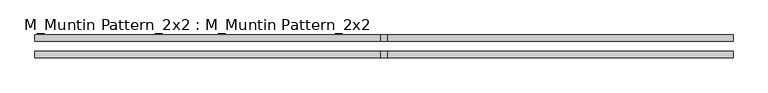
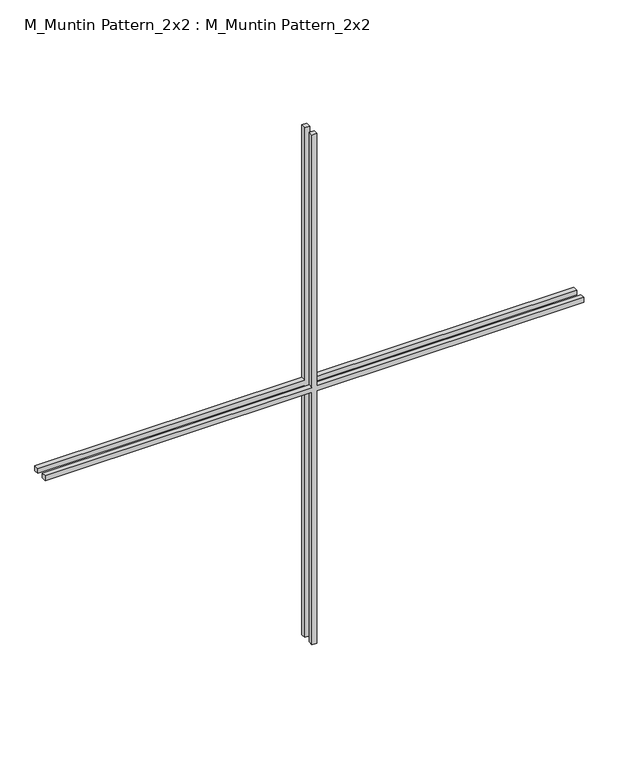
"""IFC4 building model written with IfcOpenShell, lengths in millimetres: proxy geometry, M_Muntin Pattern_2x2 : M_Muntin Pattern_2x2."""

from ifc_helpers import new_model, si_unit, frame, origin, place, context, project, spatial, polyline, outline, extrude, source, transform, mapped, element, save


def m_muntin_pattern_2x2_m_muntin_pattern_2x2_c1fd4460(model_context):
    return source(origin(), model_context, "Body", "SweptSolid", [
        extrude(outline(polyline([(686.5, -6.35), (686.5, -680.15), (673.8, -680.15), (673.8, -6.35), (0.0, -6.35), (0.0, 6.35), (673.8, 6.35), (673.8, 680.15), (686.5, 680.15), (686.5, 6.35), (1360.3, 6.35), (1360.3, -6.35), (686.5, -6.35)])), frame((0.0, 9.525, 0.0), z_axis=(0.0, 1.0, 0.0), x_axis=(0.0, 0.0, 1.0)), (0.0, 0.0, 1.0), 12.7),
        extrude(outline(polyline([(686.5, -6.35), (686.5, -680.15), (673.8, -680.15), (673.8, -6.35), (0.0, -6.35), (0.0, 6.35), (673.8, 6.35), (673.8, 680.15), (686.5, 680.15), (686.5, 6.35), (1360.3, 6.35), (1360.3, -6.35), (686.5, -6.35)])), frame((0.0, -22.225, 0.0), z_axis=(0.0, 1.0, 0.0), x_axis=(0.0, 0.0, 1.0)), (0.0, 0.0, 1.0), 12.7),
    ])


if __name__ == "__main__":
    model = new_model("IFC4")
    model_context = context("Model", 3, world=origin())
    ifc_project = project(units=[si_unit("LENGTHUNIT", "METRE", prefix="MILLI")], contexts=[model_context])
    site = spatial("IfcSite", under=ifc_project)
    building = spatial("IfcBuilding", under=site)
    placement = place(None, origin())
    m_muntin_pattern_2x2_m_muntin_pattern_2x2_shape = m_muntin_pattern_2x2_m_muntin_pattern_2x2_c1fd4460(model_context)
    element("IfcBuildingElementProxy", 1, Name="M_Muntin Pattern_2x2 : M_Muntin Pattern_2x2", ObjectType="M_Muntin Pattern_2x2 : M_Muntin Pattern_2x2", at=placement, inside=building, context=model_context, shape_type="MappedRepresentation", body=[
        mapped(m_muntin_pattern_2x2_m_muntin_pattern_2x2_shape, transform((0.0, 0.0, 0.0), x_axis=(1.0, 0.0, 0.0), y_axis=(0.0, 1.0, 0.0), z_axis=(0.0, 0.0, 1.0))),
    ])
    save(model, "model.ifc")

# Revit data of these elements
# Type "M_Muntin Pattern_2x2 : M_Muntin Pattern_2x2"
#   Width [instance default] = 3' - 11.24409"
#   Thickness = 0' - 0 1/2"
#   Height [instance default] = 3' - 11.24409"
#   Distance = 0' - 0 3/4"
#   Interior Material [instance default] = none
#   Exterior Material [instance default] = none
#   Default Elevation = 0
# Element 1 (IfcBuildingElementProxy, "M_Muntin Pattern_2x2 : M_Muntin Pattern_2x2")
#   Width = 4' - 5.55512"
#   Height = 4' - 5.55512"
#   Interior Material = Wood - Stained
#   Exterior Material = Clad - White
#   Materials on its faces: "Clad - White", "Wood - Stained"
# Materials
#   "Clad - White": class "Wood", colour RGB 242 242 238, transparency 0, Cost = 0
#   "Wood - Stained": class "Wood", colour RGB 224 178 126, transparency 0, Cost = 0
